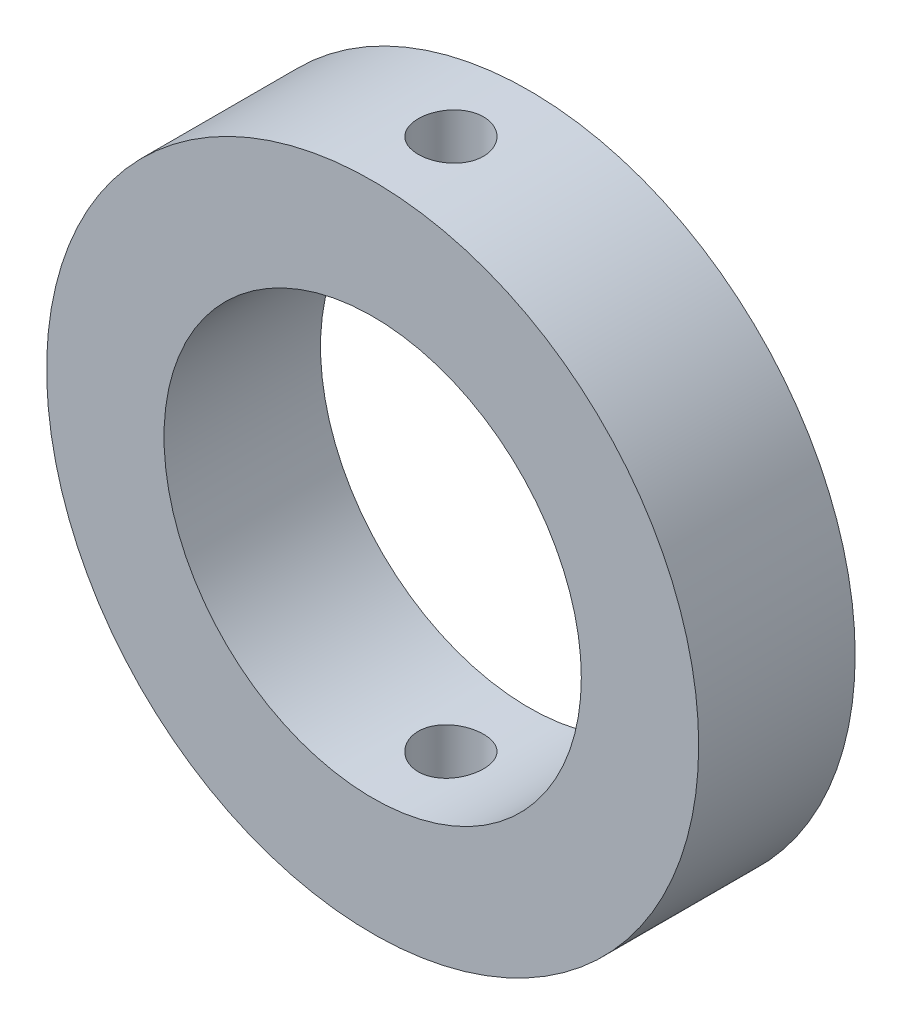
SolidWorks part; units mm, degrees
material "Plain Carbon Steel"
ref_plane "Front Plane" through (0, 0, 0) normal (0, 0, 1) x (1, 0, 0)
ref_plane "Top Plane" through (0, 0, 0) normal (0, 1, 0) x (1, 0, 0)
ref_plane "Right Plane" through (0, 0, 0) normal (1, 0, 0) x (0, 0, -1)
sketch "Collar Ring Profile" plane through (0, 0, 0) normal (0, 0, 1) x (1, 0, 0)
  circle A0 centre (0, 0) radius 16
  circle A1 centre (0, 0) radius 25
  dimension "D1" = 32
  dimension "D2" = 50
extrude "Collar Ring OD50xID32x12" add sketch "Collar Ring Profile" along normal blind 12
sketch "Cross Hole Sketch" plane through (0, 0, 0) normal (0, 1, 0) x (1, 0, 0)
  line L0 (0, 5.2702) -> (0, -15.0763) construction
  circle A0 centre (0, -6) radius 2.5
  dimension "D1" = 5
  dimension "D2" = 6
extrude "Cross Hole Ø5" cut sketch "Cross Hole Sketch" against normal mid plane 80
